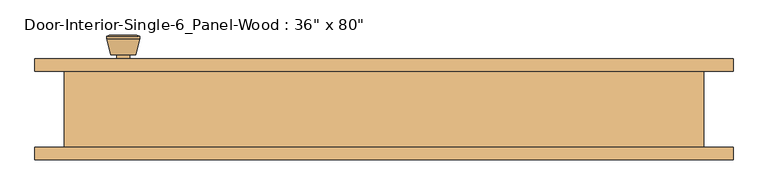
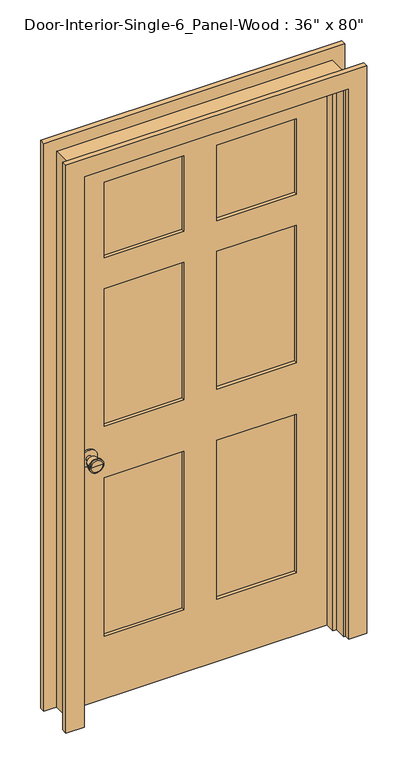
"""IFC4 building model written with IfcOpenShell, lengths in millimetres: door geometry."""

from ifc_helpers import new_model, si_unit, point, frame, frame_2d, origin, place, context, project, spatial, polyline, circle_curve, trimmed, segment, composite_curve, outline, extrude, faceted_brep, source, transform, mapped, element, save
from ifc_brep_helpers import plane_surface, cylinder_surface, revolved_surface, advanced_brep


def door_92bad2d9(model_context):
    return source(origin(), model_context, "Body", "SolidModel", [
        advanced_brep(
        [(-393.7, 13.05, 914.4), (-383.7, 13.05, 914.4), (-403.7, 13.05, 914.4), (-373.2241324, -35.95, 914.4), (-393.7, -35.95, 914.4), (-414.1758676, -35.95, 914.4), (-368.7, -34.1221319, 914.4), (-418.7, -34.1221319, 914.4), (-368.7, -30.6584537, 914.4), (-418.7, -30.6584537, 914.4), (-375.063764, -5.95, 914.4), (-412.336236, -5.95, 914.4), (-383.7, -5.95, 914.4), (-403.7, -5.95, 914.4)],
        [
            (0, 1),
            (1, 2, circle_curve(frame((-393.7, 13.05, 914.4), z_axis=(0.0, 1.0, 0.0), x_axis=(-1.0, 0.0, 0.0)), 10.0)),
            (2, 0),
            (2, 1, circle_curve(frame((-393.7, 13.05, 914.4), z_axis=(0.0, 1.0, 0.0), x_axis=(-1.0, 0.0, 0.0)), 10.0)),
            (3, 4),
            (4, 5),
            (5, 3, circle_curve(frame((-393.7, -35.95, 914.4), z_axis=(0.0, -1.0, 0.0), x_axis=(-1.0, 0.0, 0.0)), 20.4758676)),
            (3, 5, circle_curve(frame((-393.7, -35.95, 914.4), z_axis=(0.0, -1.0, 0.0), x_axis=(-1.0, 0.0, 0.0)), 20.4758676)),
            (6, 3),
            (5, 7),
            (7, 6, circle_curve(frame((-393.7, -34.1221319, 914.4), z_axis=(0.0, -1.0, 0.0), x_axis=(-1.0, 0.0, 0.0)), 25.0)),
            (6, 7, circle_curve(frame((-393.7, -34.1221319, 914.4), z_axis=(0.0, -1.0, 0.0), x_axis=(-1.0, 0.0, 0.0)), 25.0)),
            (8, 6),
            (7, 9),
            (9, 8, circle_curve(frame((-393.7, -30.6584537, 914.4), z_axis=(0.0, -1.0, 0.0), x_axis=(-1.0, 0.0, 0.0)), 25.0)),
            (8, 9, circle_curve(frame((-393.7, -30.6584537, 914.4), z_axis=(0.0, -1.0, 0.0), x_axis=(-1.0, 0.0, 0.0)), 25.0)),
            (10, 8),
            (9, 11),
            (11, 10, circle_curve(frame((-393.7, -5.95, 914.4), z_axis=(0.0, -1.0, 0.0), x_axis=(-1.0, 0.0, 0.0)), 18.636236)),
            (10, 11, circle_curve(frame((-393.7, -5.95, 914.4), z_axis=(0.0, -1.0, 0.0), x_axis=(-1.0, 0.0, 0.0)), 18.636236)),
            (12, 10),
            (11, 13),
            (13, 12, circle_curve(frame((-393.7, -5.95, 914.4), z_axis=(0.0, -1.0, 0.0), x_axis=(-1.0, 0.0, 0.0)), 10.0)),
            (12, 13, circle_curve(frame((-393.7, -5.95, 914.4), z_axis=(0.0, -1.0, 0.0), x_axis=(-1.0, 0.0, 0.0)), 10.0)),
            (1, 12),
            (13, 2),
        ],
        [
            plane_surface(frame((-393.7, 13.05, 914.4), z_axis=(0.0, 1.0, 0.0), x_axis=(-1.0, 0.0, 0.0))),
            plane_surface(frame((-393.7, -35.95, 914.4), z_axis=(0.0, -1.0, 0.0), x_axis=(-1.0, 0.0, 0.0))),
            revolved_surface(polyline([(-414.1758676, -35.95, 914.4), (-418.7, -34.1221319, 914.4)]), (-393.7, 13.05, 914.4), (0.0, 1.0, 0.0)),
            cylinder_surface(frame((-393.7, 13.05, 914.4), z_axis=(0.0, 1.0, 0.0), x_axis=(-1.0, 0.0, 0.0)), 25.0),
            revolved_surface(polyline([(-418.7, -30.6584537, 914.4), (-412.336236, -5.95, 914.4)]), (-393.7, 13.05, 914.4), (0.0, 1.0, 0.0)),
            plane_surface(frame((-393.7, -5.95, 914.4), z_axis=(0.0, 1.0, 0.0), x_axis=(-1.0, 0.0, 0.0))),
            cylinder_surface(frame((-393.7, 13.05, 914.4), z_axis=(0.0, 1.0, 0.0), x_axis=(-1.0, 0.0, 0.0)), 10.0),
        ],
        [
            (0, [[1, 2, 3]]),
            (0, [[-3, 4, -1]]),
            (1, [[5, 6, 7]]),
            (1, [[-6, -5, 8]]),
            (2, [[9, -7, 10, 11]]),
            (2, [[-10, -8, -9, 12]]),
            (3, [[13, -11, 14, 15]]),
            (3, [[-14, -12, -13, 16]]),
            (4, [[17, -15, 18, 19]]),
            (4, [[-18, -16, -17, 20]]),
            (5, [[21, -19, 22, 23]]),
            (5, [[-22, -20, -21, 24]]),
            (6, [[25, -23, 26, -2]]),
            (6, [[-26, -24, -25, -4]]),
        ],
    ),
        extrude(outline(composite_curve([segment(trimmed(circle_curve(frame_2d((914.4, -393.7)), 30.0), [point((914.4, -423.7))], [point((914.4, -363.7))], False, "CARTESIAN"), True, "CONTINUOUS"), segment(trimmed(circle_curve(frame_2d((914.4, -393.7)), 30.0), [point((914.4, -363.7))], [point((914.4, -423.7))], False, "CARTESIAN"), True, "CONTINUOUS")], self_intersect=False)), frame((0.0, 13.05, 0.0), z_axis=(0.0, 1.0, 0.0), x_axis=(0.0, 0.0, 1.0)), (0.0, 0.0, 1.0), 6.0),
        advanced_brep(
        [(-393.7, 59.975, 914.4), (-403.7, 59.975, 914.4), (-383.7, 59.975, 914.4), (-373.2241324, 108.975, 914.4), (-414.1758676, 108.975, 914.4), (-393.7, 108.975, 914.4), (-368.7, 107.1471319, 914.4), (-418.7, 107.1471319, 914.4), (-368.7, 103.6834537, 914.4), (-418.7, 103.6834537, 914.4), (-375.063764, 78.975, 914.4), (-412.336236, 78.975, 914.4), (-383.7, 78.975, 914.4), (-403.7, 78.975, 914.4)],
        [
            (0, 1),
            (1, 2, circle_curve(frame((-393.7, 59.975, 914.4), z_axis=(0.0, -1.0, 0.0), x_axis=(-1.0, 0.0, 0.0)), 10.0)),
            (2, 0),
            (2, 1, circle_curve(frame((-393.7, 59.975, 914.4), z_axis=(0.0, -1.0, 0.0), x_axis=(-1.0, 0.0, 0.0)), 10.0)),
            (3, 4, circle_curve(frame((-393.7, 108.975, 914.4), z_axis=(0.0, 1.0, 0.0), x_axis=(-1.0, 0.0, 0.0)), 20.4758676)),
            (4, 5),
            (5, 3),
            (4, 3, circle_curve(frame((-393.7, 108.975, 914.4), z_axis=(0.0, 1.0, 0.0), x_axis=(-1.0, 0.0, 0.0)), 20.4758676)),
            (6, 7, circle_curve(frame((-393.7, 107.1471319, 914.4), z_axis=(0.0, 1.0, 0.0), x_axis=(-1.0, 0.0, 0.0)), 25.0)),
            (7, 4),
            (3, 6),
            (7, 6, circle_curve(frame((-393.7, 107.1471319, 914.4), z_axis=(0.0, 1.0, 0.0), x_axis=(-1.0, 0.0, 0.0)), 25.0)),
            (8, 9, circle_curve(frame((-393.7, 103.6834537, 914.4), z_axis=(0.0, 1.0, 0.0), x_axis=(-1.0, 0.0, 0.0)), 25.0)),
            (9, 7),
            (6, 8),
            (9, 8, circle_curve(frame((-393.7, 103.6834537, 914.4), z_axis=(0.0, 1.0, 0.0), x_axis=(-1.0, 0.0, 0.0)), 25.0)),
            (10, 11, circle_curve(frame((-393.7, 78.975, 914.4), z_axis=(0.0, 1.0, 0.0), x_axis=(-1.0, 0.0, 0.0)), 18.636236)),
            (11, 9),
            (8, 10),
            (11, 10, circle_curve(frame((-393.7, 78.975, 914.4), z_axis=(0.0, 1.0, 0.0), x_axis=(-1.0, 0.0, 0.0)), 18.636236)),
            (12, 13, circle_curve(frame((-393.7, 78.975, 914.4), z_axis=(0.0, 1.0, 0.0), x_axis=(-1.0, 0.0, 0.0)), 10.0)),
            (13, 11),
            (10, 12),
            (13, 12, circle_curve(frame((-393.7, 78.975, 914.4), z_axis=(0.0, 1.0, 0.0), x_axis=(-1.0, 0.0, 0.0)), 10.0)),
            (1, 13),
            (12, 2),
        ],
        [
            plane_surface(frame((-393.7, 59.975, 914.4), z_axis=(0.0, -1.0, 0.0), x_axis=(-1.0, 0.0, 0.0))),
            plane_surface(frame((-393.7, 108.975, 914.4), z_axis=(0.0, 1.0, 0.0), x_axis=(-1.0, 0.0, 0.0))),
            revolved_surface(polyline([(-414.1758676, 108.975, 914.4), (-418.7, 107.1471319, 914.4)]), (-393.7, 59.975, 914.4), (0.0, -1.0, 0.0)),
            cylinder_surface(frame((-393.7, 59.975, 914.4), z_axis=(0.0, -1.0, 0.0), x_axis=(-1.0, 0.0, 0.0)), 25.0),
            revolved_surface(polyline([(-418.7, 103.6834537, 914.4), (-412.336236, 78.975, 914.4)]), (-393.7, 59.975, 914.4), (0.0, -1.0, 0.0)),
            plane_surface(frame((-393.7, 78.975, 914.4), z_axis=(0.0, -1.0, 0.0), x_axis=(-1.0, 0.0, 0.0))),
            cylinder_surface(frame((-393.7, 59.975, 914.4), z_axis=(0.0, -1.0, 0.0), x_axis=(-1.0, 0.0, 0.0)), 10.0),
        ],
        [
            (0, [[1, 2, 3]]),
            (0, [[-3, 4, -1]]),
            (1, [[5, 6, 7]]),
            (1, [[8, -7, -6]]),
            (2, [[9, 10, -5, 11]]),
            (2, [[12, -11, -8, -10]]),
            (3, [[13, 14, -9, 15]]),
            (3, [[16, -15, -12, -14]]),
            (4, [[17, 18, -13, 19]]),
            (4, [[20, -19, -16, -18]]),
            (5, [[21, 22, -17, 23]]),
            (5, [[24, -23, -20, -22]]),
            (6, [[-2, 25, -21, 26]]),
            (6, [[-4, -26, -24, -25]]),
        ],
    ),
        extrude(outline(composite_curve([segment(trimmed(circle_curve(frame_2d((914.4, -393.7)), 30.0), [point((914.4, -423.7))], [point((914.4, -363.7))], False, "CARTESIAN"), True, "CONTINUOUS"), segment(trimmed(circle_curve(frame_2d((914.4, -393.7)), 30.0), [point((914.4, -363.7))], [point((914.4, -423.7))], False, "CARTESIAN"), True, "CONTINUOUS")], self_intersect=False)), frame((0.0, 53.975, 0.0), z_axis=(0.0, 1.0, 0.0), x_axis=(0.0, 0.0, 1.0)), (0.0, 0.0, 1.0), 6.0),
        faceted_brep([(482.6, 53.975, 0.0), (482.6, -60.325, 0.0), (457.2, -60.325, 0.0), (457.2, -15.875, 0.0), (444.5, -15.875, 0.0), (444.5, 19.05, 0.0), (457.2, 19.05, 0.0), (457.2, 53.975, 0.0), (482.6, 53.975, 2057.4), (482.6, -60.325, 2057.4), (-482.6, -60.325, 2057.4), (-482.6, -60.325, 0.0), (-457.2, -60.325, 0.0), (-457.2, -60.325, 2032.0), (457.2, -60.325, 2032.0), (457.2, -15.875, 2032.0), (-457.2, -15.875, 2032.0), (-457.2, -15.875, 0.0), (-444.5, -15.875, 0.0), (-444.5, -15.875, 2019.3), (444.5, -15.875, 2019.3), (444.5, 19.05, 2019.3), (-444.5, 19.05, 2019.3), (-444.5, 19.05, 0.0), (-457.2, 19.05, 0.0), (-457.2, 19.05, 2032.0), (457.2, 19.05, 2032.0), (457.2, 53.975, 2032.0), (-457.2, 53.975, 2032.0), (-457.2, 53.975, 0.0), (-482.6, 53.975, 0.0), (-482.6, 53.975, 2057.4)], [[[0, 1, 2, 3, 4, 5, 6, 7]], [[1, 0, 8, 9]], [[2, 1, 9, 10, 11, 12, 13, 14]], [[3, 2, 14, 15]], [[4, 3, 15, 16, 17, 18, 19, 20]], [[5, 4, 20, 21]], [[6, 5, 21, 22, 23, 24, 25, 26]], [[7, 6, 26, 27]], [[0, 7, 27, 28, 29, 30, 31, 8]], [[9, 8, 31, 10]], [[15, 14, 13, 16]], [[21, 20, 19, 22]], [[27, 26, 25, 28]], [[30, 29, 24, 23, 18, 17, 12, 11]], [[10, 31, 30, 11]], [[16, 13, 12, 17]], [[22, 19, 18, 23]], [[28, 25, 24, 29]]]),
        extrude(outline(polyline([(2032.0, -457.2), (0.0, -457.2), (0.0, 457.2), (2032.0, 457.2), (2032.0, -457.2)]), holes=[polyline([(1912.9375, 57.15), (1912.9375, 336.55), (1633.5375, 336.55), (1633.5375, 57.15), (1912.9375, 57.15)]), polyline([(1519.2375, 336.55), (1009.65, 336.55), (1009.65, 57.15), (1519.2375, 57.15), (1519.2375, 336.55)]), polyline([(1009.65, -57.15), (1009.65, -336.55), (1519.2375, -336.55), (1519.2375, -57.15), (1009.65, -57.15)]), polyline([(1633.5375, -336.55), (1912.9375, -336.55), (1912.9375, -57.15), (1633.5375, -57.15), (1633.5375, -336.55)]), polyline([(819.15, 57.15), (819.15, 336.55), (231.775, 336.55), (231.775, 57.15), (819.15, 57.15)]), polyline([(231.775, -57.15), (231.775, -336.55), (819.15, -336.55), (819.15, -57.15), (231.775, -57.15)])]), frame((0.0, 19.05, 0.0), z_axis=(0.0, 1.0, 0.0), x_axis=(0.0, 0.0, 1.0)), (0.0, 0.0, 1.0), 34.925),
        extrude(outline(polyline([(336.55, 30.6916667), (57.15, 30.6916667), (57.15, 42.3333333), (336.55, 42.3333333), (336.55, 30.6916667)])), frame((0.0, 0.0, 1633.5375), z_axis=(0.0, 0.0, 1.0), x_axis=(1.0, 0.0, 0.0)), (0.0, 0.0, 1.0), 279.4),
        extrude(outline(polyline([(336.55, 30.6916667), (57.15, 30.6916667), (57.15, 42.3333333), (336.55, 42.3333333), (336.55, 30.6916667)])), frame((0.0, 0.0, 1009.65), z_axis=(0.0, 0.0, 1.0), x_axis=(1.0, 0.0, 0.0)), (0.0, 0.0, 1.0), 509.5875),
        extrude(outline(polyline([(-57.15, 30.6916667), (-336.55, 30.6916667), (-336.55, 42.3333333), (-57.15, 42.3333333), (-57.15, 30.6916667)])), frame((0.0, 0.0, 1009.65), z_axis=(0.0, 0.0, 1.0), x_axis=(1.0, 0.0, 0.0)), (0.0, 0.0, 1.0), 509.5875),
        extrude(outline(polyline([(-57.15, 30.6916667), (-336.55, 30.6916667), (-336.55, 42.3333333), (-57.15, 42.3333333), (-57.15, 30.6916667)])), frame((0.0, 0.0, 1633.5375), z_axis=(0.0, 0.0, 1.0), x_axis=(1.0, 0.0, 0.0)), (0.0, 0.0, 1.0), 279.4),
        extrude(outline(polyline([(336.55, 30.6916667), (57.15, 30.6916667), (57.15, 42.3333333), (336.55, 42.3333333), (336.55, 30.6916667)])), frame((0.0, 0.0, 231.775), z_axis=(0.0, 0.0, 1.0), x_axis=(1.0, 0.0, 0.0)), (0.0, 0.0, 1.0), 587.375),
        extrude(outline(polyline([(-57.15, 30.6916667), (-336.55, 30.6916667), (-336.55, 42.3333333), (-57.15, 42.3333333), (-57.15, 30.6916667)])), frame((0.0, 0.0, 231.775), z_axis=(0.0, 0.0, 1.0), x_axis=(1.0, 0.0, 0.0)), (0.0, 0.0, 1.0), 587.375),
        extrude(outline(polyline([(0.0, 463.55), (0.0, 527.05), (2101.85, 527.05), (2101.85, -527.05), (0.0, -527.05), (0.0, -463.55), (2038.35, -463.55), (2038.35, 463.55), (0.0, 463.55)])), frame((0.0, 53.975, 0.0), z_axis=(0.0, 1.0, 0.0), x_axis=(0.0, 0.0, 1.0)), (0.0, 0.0, 1.0), 19.05),
        extrude(outline(polyline([(0.0, 463.55), (0.0, 527.05), (2101.85, 527.05), (2101.85, -527.05), (0.0, -527.05), (0.0, -463.55), (2038.35, -463.55), (2038.35, 463.55), (0.0, 463.55)])), frame((0.0, -79.375, 0.0), z_axis=(0.0, 1.0, 0.0), x_axis=(0.0, 0.0, 1.0)), (0.0, 0.0, 1.0), 19.05),
    ])


if __name__ == "__main__":
    model = new_model("IFC4")
    model_context = context("Model", 3, world=origin())
    ifc_project = project(units=[si_unit("LENGTHUNIT", "METRE", prefix="MILLI")], contexts=[model_context])
    site = spatial("IfcSite", under=ifc_project)
    building = spatial("IfcBuilding", under=site)
    placement = place(None, origin())
    door_shape = door_92bad2d9(model_context)
    element("IfcDoor", 1, ObjectType="Door-Interior-Single-6_Panel-Wood : 36\" x 80\"", at=placement, inside=building, context=model_context, shape_type="MappedRepresentation", body=[
        mapped(door_shape, transform((0.0, 0.0, 0.0), x_axis=(1.0, 0.0, 0.0), y_axis=(0.0, 1.0, 0.0), z_axis=(0.0, 0.0, 1.0))),
    ])
    save(model, "model.ifc")

# Revit data of these elements
# Type "Door-Interior-Single-6_Panel-Wood : 36\" x 80\""
#   Type Mark = "10"
#   Assembly Code = "C1020300"
#   Analytic Construction = "Wooden"
#   Top Rail = 0' - 4 11/16"
#   Top Panel = 0' - 11"
#   Thickness = 0' - 1 3/8"
#   Thermal Resistance (R) = 2.5876 (h·ft²·°F)/BTU
#   Swing Angle [instance default] = 90.00°
#   Stiles = 0' - 4 3/4"
#   Rough Width = 3' - 2"
#   Rough Height = 6' - 9"
#   Mullion = 0' - 4 1/2"
#   Lock Rail = 0' - 7 1/2"
#   Intermediate Rail = 0' - 4 1/2"
#   Height = 6' - 8"
#   Width = 3' - 0"
#   Heat Transfer Coefficient (U) = 0.3865 BTU/(h·ft²·°F)
#   Bottom Rail = 0' - 9 1/8"
#   Trim Material = Cherry
#   Panel Material = Cherry
#   Frame Material = Cherry
#   Door Handle Material = Aluminum
#   Visual Light Transmittance = 0
#   Solar Heat Gain Coefficient = 0
#   Wall Closure = (empty or 0)
#   Function = (empty or 0)
# Element 1 (IfcDoor, "Door-Interior-Single-6_Panel-Wood : 36\" x 80\"")
#   Materials on its faces: "Cherry", "Aluminum"
# Materials
#   "Cherry": class "Wood", colour RGB 226 177 128, transparency 0, Description = "Prunus Serotina", Cost = 0
#   "Aluminum": class "Metal", colour RGB 247 247 247, transparency 0, Description = "Aluminum 6061", Cost = 0
